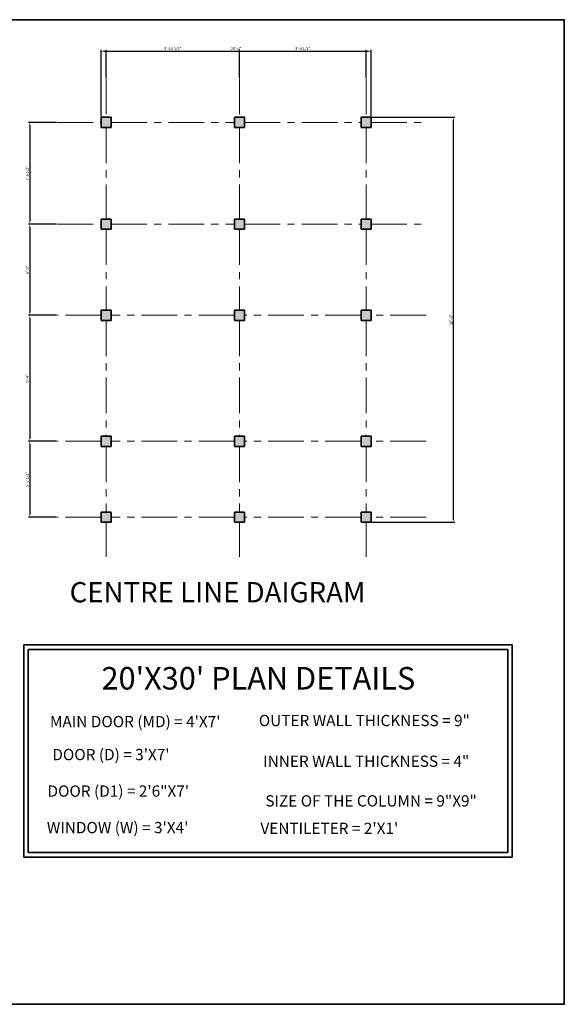
# Model space of a CAD drawing. Units: inches. Extents: x 2150 to 10686, y 1035 to 5077.
# Tile 9 of 12: x 6517 to 7001, y 4201 to 5077. Entities that reach past the tile are written whole.
import ezdxf

# ---------------------------------------------------------------- set-up
doc = ezdxf.new("R2010")
doc.units = ezdxf.units.IN
doc.linetypes.add('CENTER', pattern=[50.8, 31.75, -6.35, 6.35, -6.35])
for name, color, linetype, lineweight in [('A-ANNO-DIMS', 2, 'Continuous', 18), ('A-ANNO-TEXT', 2, 'Continuous', 18), ('A-ANNO-TITL', 3, 'Continuous', 35), ('A-ANNO-TTLB', 7, 'Continuous', 35), ('A-COLS', 7, 'Continuous', 35), ('A-COLS-PATT', 8, 'Continuous', 13), ('A-GRID', 1, 'CENTER', 18)]:
    doc.layers.add(name, color=color, linetype=linetype, lineweight=lineweight)
doc.styles.get("Standard").update_dxf_attribs({"font": 'arial.ttf'})
doc.dimstyles.new('ISO-25', dxfattribs={"dimtxt": 2.5, "dimasz": 2.5, "dimexe": 1.25, "dimexo": 0.625, "dimtad": 1, "dimdec": 0, "dimlunit": 3, "dimtxsty": 'Standard', "dimcen": 2.5, "dimadec": 0, "dimazin": 0, "dimtfac": 1, "dimtdec": 0, "dimtmove": 0, "dimatfit": 3, "dimfxl": 1, "dimarcsym": 0})

# ---------------------------------------------------------------- blocks, each defined once
blk = doc.blocks.new('COL-SQUARE-9IN')
for p, q in [((0, 9), (9, 9)), ((0, 0), (0, 9)), ((9, 9), (9, 0)), ((9, 0), (0, 0))]:
    blk.add_line(p, q)
blk = doc.blocks.new('*D95')
at = {"layer": 'A-ANNO-DIMS', "color": 0, "lineweight": -2, "transparency": 16777216}
for p, q in [((6594.09, 5024.87), (6594.09, 5049.94)), ((6596.59, 5048.69), (6710.09, 5048.69)), ((6712.59, 5024.87), (6712.59, 5049.94))]:
    blk.add_line(p, q, dxfattribs=at)
at = {"layer": 'A-ANNO-DIMS', "color": 0, "transparency": 16777216}
for points in [[(6596.59, 5049.11), (6596.59, 5048.27), (6594.09, 5048.69)], [(6710.09, 5049.11), (6710.09, 5048.27), (6712.59, 5048.69)]]:
    blk.add_solid(points, dxfattribs=at)
at = {"layer": 'Defpoints', "color": 0, "transparency": 16777216}
for p in [(6712.59, 5048.69), (6594.09, 5024.24), (6712.59, 5024.24)]:
    blk.add_point(p, dxfattribs=at)
at = {"layer": 'A-ANNO-DIMS', "color": 0, "transparency": 16777216, "insert": (6653.34, 5050.61), "char_height": 2.5, "attachment_point": 5}
blk.add_mtext('9\'-10 1/2"', dxfattribs=at)
blk = doc.blocks.new('*D96')
at = {"layer": 'A-ANNO-DIMS', "color": 0, "lineweight": -2, "transparency": 16777216}
for p, q in [((6712.59, 5024.87), (6712.59, 5049.94)), ((6715.09, 5048.69), (6822.59, 5048.69)), ((6825.09, 5024.87), (6825.09, 5049.94))]:
    blk.add_line(p, q, dxfattribs=at)
at = {"layer": 'A-ANNO-DIMS', "color": 0, "transparency": 16777216}
for points in [[(6715.09, 5049.11), (6715.09, 5048.27), (6712.59, 5048.69)], [(6822.59, 5049.11), (6822.59, 5048.27), (6825.09, 5048.69)]]:
    blk.add_solid(points, dxfattribs=at)
at = {"layer": 'Defpoints', "color": 0, "transparency": 16777216}
for p in [(6825.09, 5048.69), (6712.59, 5024.24), (6825.09, 5024.24)]:
    blk.add_point(p, dxfattribs=at)
at = {"layer": 'A-ANNO-DIMS', "color": 0, "transparency": 16777216, "insert": (6768.84, 5050.61), "char_height": 2.5, "attachment_point": 5}
blk.add_mtext('9\'-4 1/2"', dxfattribs=at)
blk = doc.blocks.new('*D97')
at = {"layer": 'A-ANNO-DIMS', "color": 0, "lineweight": -2, "transparency": 16777216}
for p, q in [((6550.01, 4985.32), (6524.94, 4985.32)), ((6526.19, 4982.82), (6526.19, 4897.32)), ((6550.01, 4894.82), (6524.94, 4894.82))]:
    blk.add_line(p, q, dxfattribs=at)
at = {"layer": 'A-ANNO-DIMS', "color": 0, "transparency": 16777216}
for points in [[(6525.77, 4982.82), (6526.6, 4982.82), (6526.19, 4985.32)], [(6525.77, 4897.32), (6526.6, 4897.32), (6526.19, 4894.82)]]:
    blk.add_solid(points, dxfattribs=at)
at = {"layer": 'Defpoints', "color": 0, "transparency": 16777216}
for p in [(6550.64, 4985.32), (6526.19, 4894.82), (6550.64, 4894.82)]:
    blk.add_point(p, dxfattribs=at)
at = {"layer": 'A-ANNO-DIMS', "color": 0, "transparency": 16777216, "insert": (6524.27, 4940.07), "char_height": 2.5, "attachment_point": 5, "rotation": 90}
blk.add_mtext('7\'-6 1/2"', dxfattribs=at)
blk = doc.blocks.new('*D98')
at = {"layer": 'A-ANNO-DIMS', "color": 0, "lineweight": -2, "transparency": 16777216}
for p, q in [((6550.01, 4894.82), (6524.94, 4894.82)), ((6526.19, 4892.32), (6526.19, 4816.32)), ((6550.01, 4813.82), (6524.94, 4813.82))]:
    blk.add_line(p, q, dxfattribs=at)
at = {"layer": 'A-ANNO-DIMS', "color": 0, "transparency": 16777216}
for points in [[(6525.77, 4892.32), (6526.6, 4892.32), (6526.19, 4894.82)], [(6525.77, 4816.32), (6526.6, 4816.32), (6526.19, 4813.82)]]:
    blk.add_solid(points, dxfattribs=at)
at = {"layer": 'Defpoints', "color": 0, "transparency": 16777216}
for p in [(6550.64, 4894.82), (6526.19, 4813.82), (6550.64, 4813.82)]:
    blk.add_point(p, dxfattribs=at)
at = {"layer": 'A-ANNO-DIMS', "color": 0, "transparency": 16777216, "insert": (6524.29, 4854.32), "char_height": 2.5, "attachment_point": 5, "rotation": 90}
blk.add_mtext('6\'-9"', dxfattribs=at)
blk = doc.blocks.new('*D99')
at = {"layer": 'A-ANNO-DIMS', "color": 0, "lineweight": -2, "transparency": 16777216}
for p, q in [((6550.01, 4813.82), (6524.94, 4813.82)), ((6526.19, 4811.32), (6526.19, 4704.32)), ((6550.01, 4701.82), (6524.94, 4701.82))]:
    blk.add_line(p, q, dxfattribs=at)
at = {"layer": 'A-ANNO-DIMS', "color": 0, "transparency": 16777216}
for points in [[(6525.77, 4811.32), (6526.6, 4811.32), (6526.19, 4813.82)], [(6525.77, 4704.32), (6526.6, 4704.32), (6526.19, 4701.82)]]:
    blk.add_solid(points, dxfattribs=at)
at = {"layer": 'Defpoints', "color": 0, "transparency": 16777216}
for p in [(6550.64, 4813.82), (6526.19, 4701.82), (6550.64, 4701.82)]:
    blk.add_point(p, dxfattribs=at)
at = {"layer": 'A-ANNO-DIMS', "color": 0, "transparency": 16777216, "insert": (6524.29, 4757.82), "char_height": 2.5, "attachment_point": 5, "rotation": 90}
blk.add_mtext('9\'-4"', dxfattribs=at)
blk = doc.blocks.new('*D100')
at = {"layer": 'A-ANNO-DIMS', "color": 0, "lineweight": -2, "transparency": 16777216}
for p, q in [((6550.01, 4701.82), (6524.94, 4701.82)), ((6526.19, 4699.32), (6526.19, 4636.82)), ((6550.01, 4634.32), (6524.94, 4634.32))]:
    blk.add_line(p, q, dxfattribs=at)
at = {"layer": 'A-ANNO-DIMS', "color": 0, "transparency": 16777216}
for points in [[(6525.77, 4699.32), (6526.6, 4699.32), (6526.19, 4701.82)], [(6525.77, 4636.82), (6526.6, 4636.82), (6526.19, 4634.32)]]:
    blk.add_solid(points, dxfattribs=at)
at = {"layer": 'Defpoints', "color": 0, "transparency": 16777216}
for p in [(6550.64, 4701.82), (6526.19, 4634.32), (6550.64, 4634.32)]:
    blk.add_point(p, dxfattribs=at)
at = {"layer": 'A-ANNO-DIMS', "color": 0, "transparency": 16777216, "insert": (6524.27, 4668.07), "char_height": 2.5, "attachment_point": 5, "rotation": 90}
blk.add_mtext('5\'-7 1/2"', dxfattribs=at)
blk = doc.blocks.new('*D101')
at = {"layer": 'A-ANNO-DIMS', "color": 0, "lineweight": -2, "transparency": 16777216}
for p, q in [((6589.59, 4990.45), (6589.59, 5049.94)), ((6592.09, 5048.69), (6827.09, 5048.69)), ((6829.59, 4990.45), (6829.59, 5049.94))]:
    blk.add_line(p, q, dxfattribs=at)
at = {"layer": 'A-ANNO-DIMS', "color": 0, "transparency": 16777216}
for points in [[(6592.09, 5049.11), (6592.09, 5048.27), (6589.59, 5048.69)], [(6827.09, 5049.11), (6827.09, 5048.27), (6829.59, 5048.69)]]:
    blk.add_solid(points, dxfattribs=at)
at = {"layer": 'Defpoints', "color": 0, "transparency": 16777216}
for p in [(6829.59, 5048.69), (6589.59, 4989.82), (6829.59, 4989.82)]:
    blk.add_point(p, dxfattribs=at)
at = {"layer": 'A-ANNO-DIMS', "color": 0, "transparency": 16777216, "insert": (6709.59, 5050.59), "char_height": 2.5, "attachment_point": 5}
blk.add_mtext('20\'-0"', dxfattribs=at)
blk = doc.blocks.new('*D102')
at = {"layer": 'A-ANNO-DIMS', "color": 0, "lineweight": -2, "transparency": 16777216}
for p, q in [((6830.22, 4989.82), (6904.07, 4989.82)), ((6902.82, 4632.32), (6902.82, 4987.32)), ((6830.22, 4629.82), (6904.07, 4629.82))]:
    blk.add_line(p, q, dxfattribs=at)
at = {"layer": 'A-ANNO-DIMS', "color": 0, "transparency": 16777216}
for points in [[(6902.41, 4987.32), (6903.24, 4987.32), (6902.82, 4989.82)], [(6902.41, 4632.32), (6903.24, 4632.32), (6902.82, 4629.82)]]:
    blk.add_solid(points, dxfattribs=at)
at = {"layer": 'Defpoints', "color": 0, "transparency": 16777216}
for p in [(6829.59, 4989.82), (6902.82, 4989.82), (6829.59, 4629.82)]:
    blk.add_point(p, dxfattribs=at)
at = {"layer": 'A-ANNO-DIMS', "color": 0, "transparency": 16777216, "insert": (6900.92, 4809.82), "char_height": 2.5, "attachment_point": 5, "rotation": 90}
blk.add_mtext('30\'-0"', dxfattribs=at)

msp = doc.modelspace()

# ---------------------------------------------------------------- hatches: boundary and pattern name
at = {"layer": 'A-COLS-PATT'}
h = msp.add_hatch(color=256, dxfattribs=at)
h.dxf.hatch_style = 1
h.paths.add_polyline_path([(6598.59, 4629.82), (6598.59, 4638.82), (6589.59, 4638.82), (6589.59, 4629.82)])
h.paths.add_polyline_path([(6717.09, 4638.82), (6708.09, 4638.82), (6708.09, 4629.82), (6717.09, 4629.82)])
h.paths.add_polyline_path([(6820.59, 4638.82), (6820.59, 4629.82), (6829.59, 4629.82), (6829.59, 4638.82)])
h.paths.add_polyline_path([(6829.59, 4706.32), (6820.59, 4706.32), (6820.59, 4697.32), (6829.59, 4697.32)])
h.paths.add_polyline_path([(6708.09, 4706.32), (6708.09, 4697.32), (6717.09, 4697.32), (6717.09, 4706.32)])
h.paths.add_polyline_path([(6589.59, 4697.32), (6598.59, 4697.32), (6598.59, 4706.32), (6589.59, 4706.32)])
h.paths.add_polyline_path([(6598.59, 4809.32), (6598.59, 4818.32), (6589.59, 4818.32), (6589.59, 4809.32)])
h.paths.add_polyline_path([(6717.09, 4818.32), (6708.09, 4818.32), (6708.09, 4809.32), (6717.09, 4809.32)])
h.paths.add_polyline_path([(6820.59, 4818.32), (6820.59, 4809.32), (6829.59, 4809.32), (6829.59, 4818.32)])
h.paths.add_polyline_path([(6820.59, 4899.32), (6820.59, 4890.32), (6829.59, 4890.32), (6829.59, 4899.32)])
h.paths.add_polyline_path([(6717.09, 4899.32), (6708.09, 4899.32), (6708.09, 4890.32), (6717.09, 4890.32)])
h.paths.add_polyline_path([(6598.59, 4890.32), (6598.59, 4899.32), (6589.59, 4899.32), (6589.59, 4890.32)])
h.paths.add_polyline_path([(6708.09, 4989.82), (6708.09, 4980.82), (6717.09, 4980.82), (6717.09, 4989.82)])
h.paths.add_polyline_path([(6820.59, 4980.82), (6829.59, 4980.82), (6829.59, 4989.82), (6820.59, 4989.82)])
h.paths.add_polyline_path([(6598.59, 4989.82), (6589.59, 4989.82), (6589.59, 4980.82), (6598.59, 4980.82)])

# ---------------------------------------------------------------- linework, layer by layer
at = {"layer": 'A-ANNO-TTLB'}
for points in [[(6112.69, 5076.61), (7001.25, 5076.61), (7001.25, 4201.35), (6112.69, 4201.35)], [(6520.9, 4520.88), (6954.97, 4520.88), (6954.97, 4332.28), (6520.9, 4332.28)], [(6524.9, 4516.88), (6950.97, 4516.88), (6950.97, 4336.28), (6524.9, 4336.28)]]:
    msp.add_lwpolyline(points, close=True, dxfattribs=at)
at = {"layer": 'A-COLS'}
msp.add_line((6710.59, 4980.82), (6714.59, 4980.82), dxfattribs=at)
at = {"layer": 'A-GRID'}
for p, q in [((6594.09, 5024.24), (6594.09, 4989.82)), ((6712.59, 5024.24), (6712.59, 4989.82)), ((6825.09, 5024.24), (6825.09, 4989.82)), ((6550.64, 4985.32), (6589.59, 4985.32)), ((6594.09, 4980.82), (6594.09, 4899.32)), ((6598.59, 4985.32), (6708.09, 4985.32)), ((6712.59, 4980.82), (6712.59, 4899.32)), ((6717.09, 4985.32), (6820.59, 4985.32)), ((6825.09, 4980.82), (6825.09, 4899.32)), ((6829.59, 4985.32), (6878.37, 4985.32)), ((6550.64, 4894.82), (6589.59, 4894.82)), ((6598.59, 4894.82), (6708.09, 4894.82)), ((6717.09, 4894.82), (6820.59, 4894.82)), ((6829.59, 4894.82), (6878.37, 4894.82)), ((6594.09, 4890.32), (6594.09, 4818.32)), ((6712.59, 4890.32), (6712.59, 4818.32)), ((6825.09, 4890.32), (6825.09, 4818.32)), ((6589.59, 4813.82), (6550.64, 4813.82)), ((6594.09, 4809.32), (6594.09, 4706.32)), ((6708.09, 4813.82), (6598.59, 4813.82)), ((6712.59, 4809.32), (6712.59, 4706.32)), ((6820.59, 4813.82), (6717.09, 4813.82)), ((6825.09, 4809.32), (6825.09, 4706.32)), ((6878.37, 4813.82), (6829.59, 4813.82)), ((6589.59, 4701.82), (6550.64, 4701.82)), ((6708.09, 4701.82), (6598.59, 4701.82)), ((6820.59, 4701.82), (6717.09, 4701.82)), ((6878.37, 4701.82), (6829.59, 4701.82)), ((6594.09, 4697.32), (6594.09, 4638.82)), ((6712.59, 4697.32), (6712.59, 4638.82)), ((6825.09, 4697.32), (6825.09, 4638.82)), ((6589.59, 4634.32), (6550.64, 4634.32)), ((6708.09, 4634.32), (6598.59, 4634.32)), ((6820.59, 4634.32), (6717.09, 4634.32)), ((6878.37, 4634.32), (6829.59, 4634.32)), ((6594.09, 4629.82), (6594.09, 4599.16)), ((6712.59, 4629.82), (6712.59, 4599.16)), ((6825.09, 4629.82), (6825.09, 4599.16))]:
    msp.add_line(p, q, dxfattribs=at)

# ---------------------------------------------------------------- block references
at = {"layer": 'A-COLS'}
for p in [(6589.59, 4980.82), (6708.09, 4980.82), (6820.59, 4980.82), (6589.59, 4890.32), (6708.09, 4890.32), (6820.59, 4890.32), (6589.59, 4809.32), (6708.09, 4809.32), (6820.59, 4809.32), (6589.59, 4697.32), (6708.09, 4697.32), (6820.59, 4697.32), (6589.59, 4629.82), (6708.09, 4629.82), (6820.59, 4629.82)]:
    msp.add_blockref('COL-SQUARE-9IN', p, dxfattribs=at)

# ---------------------------------------------------------------- texts
at = {"layer": 'A-ANNO-TEXT', "char_height": 10, "attachment_point": 1}
for s, width, insert in [("MAIN DOOR (MD) = 4'X7'", 1046.29, (6544.15, 4457.65)), ('OUTER WALL THICKNESS = 9"', 376.8496, (6729.78, 4458.61)), ("DOOR (D) = 3'X7'", 304.0135, (6546.25, 4428.36)), ('INNER WALL THICKNESS = 4"', 229.9749, (6733.64, 4422.42)), ('DOOR (D1) = 2\'6"X7\'', 293.9753, (6541.95, 4395.9)), ('SIZE OF THE COLUMN = 9"X9"', 272.4913, (6735.57, 4387.19)), ("WINDOW (W) = 3'X4'", 195.37, (6541.35, 4363.45)), ("VENTILETER = 2'X1'", 234.9271, (6731.18, 4362.79))]:
    msp.add_mtext_dynamic_manual_height_columns(s, width=width, gutter_width=12.5, heights=[0], dxfattribs=dict(at, insert=insert))
at = {"layer": 'A-ANNO-TITL', "attachment_point": 1}
for s, width, insert, char_height in [('CENTRE LINE DAIGRAM', 397.1101, (6561.62, 4576.68), 18), ("20'X30' PLAN DETAILS", 660.3294, (6589.94, 4501.17), 20)]:
    msp.add_mtext_dynamic_manual_height_columns(s, width=width, gutter_width=12.5, heights=[0], dxfattribs=dict(at, insert=insert, char_height=char_height))

# ---------------------------------------------------------------- dimensions: what is measured, and where the dimension line sits
at = {"layer": 'A-ANNO-DIMS'}
for base, p1, p2, picture, middle in [((6829.59, 5048.69), (6589.59, 4989.82), (6829.59, 4989.82), '*D101', (6709.59, 5050.59)), ((6712.59, 5048.69), (6594.09, 5024.24), (6712.59, 5024.24), '*D95', (6653.34, 5050.61)), ((6825.09, 5048.69), (6712.59, 5024.24), (6825.09, 5024.24), '*D96', (6768.84, 5050.61))]:
    dim = msp.add_linear_dim(base=base, p1=p1, p2=p2, dimstyle='ISO-25', override={"dimdec": 1, "dimlfac": 1, "dimrnd": 0, "dimzin": 1, "dimdsep": 46, "dimlunit": 4, "dimfrac": 2}, dxfattribs=at)
    dim.commit()
    dim.dimension.update_dxf_attribs({"geometry": picture, "text_midpoint": middle})
for base, p1, p2, picture, middle in [((6902.82, 4989.82), (6829.59, 4629.82), (6829.59, 4989.82), '*D102', (6900.92, 4809.82)), ((6526.19, 4894.82), (6550.64, 4985.32), (6550.64, 4894.82), '*D97', (6524.27, 4940.07)), ((6526.19, 4813.82), (6550.64, 4894.82), (6550.64, 4813.82), '*D98', (6524.29, 4854.32)), ((6526.19, 4701.82), (6550.64, 4813.82), (6550.64, 4701.82), '*D99', (6524.29, 4757.82)), ((6526.19, 4634.32), (6550.64, 4701.82), (6550.64, 4634.32), '*D100', (6524.27, 4668.07))]:
    dim = msp.add_linear_dim(base=base, p1=p1, p2=p2, angle=90, dimstyle='ISO-25', override={"dimdec": 1, "dimlfac": 1, "dimrnd": 0, "dimzin": 1, "dimdsep": 46, "dimlunit": 4, "dimfrac": 2}, dxfattribs=at)
    dim.commit()
    dim.dimension.update_dxf_attribs({"geometry": picture, "text_midpoint": middle})

doc.saveas('drawing.dxf')
